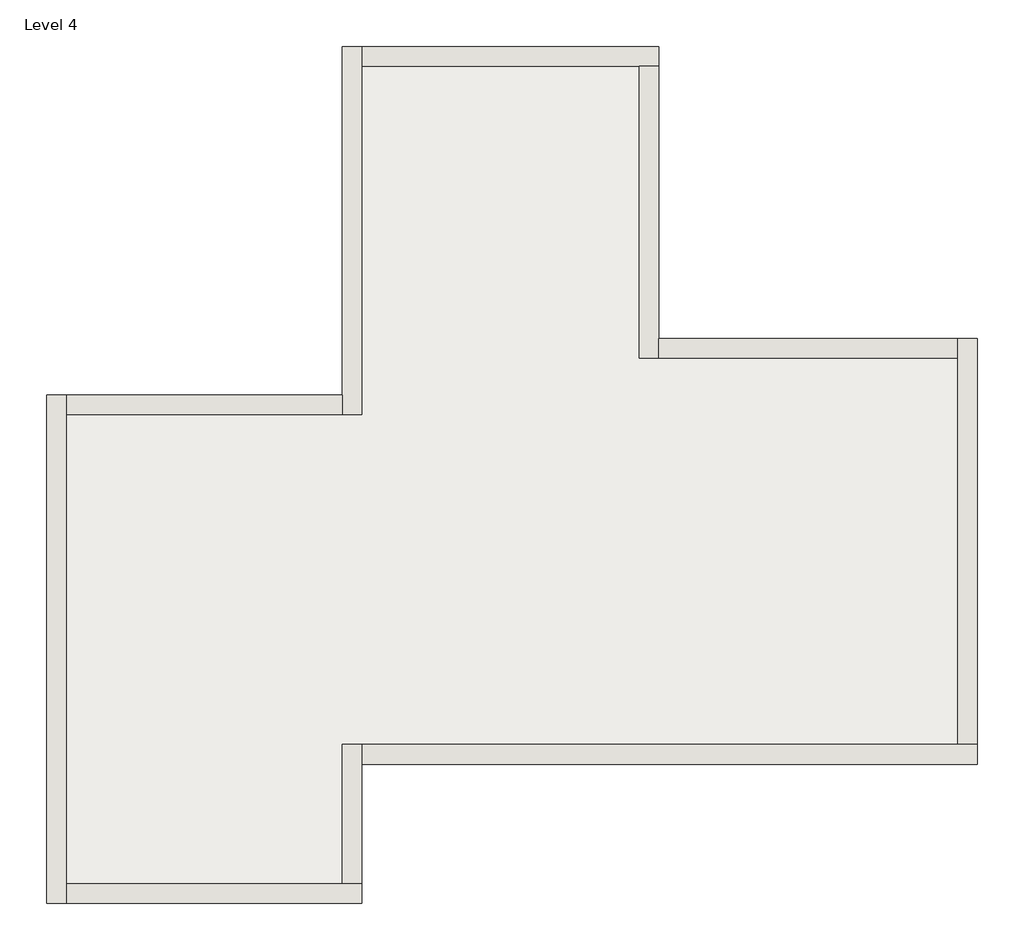
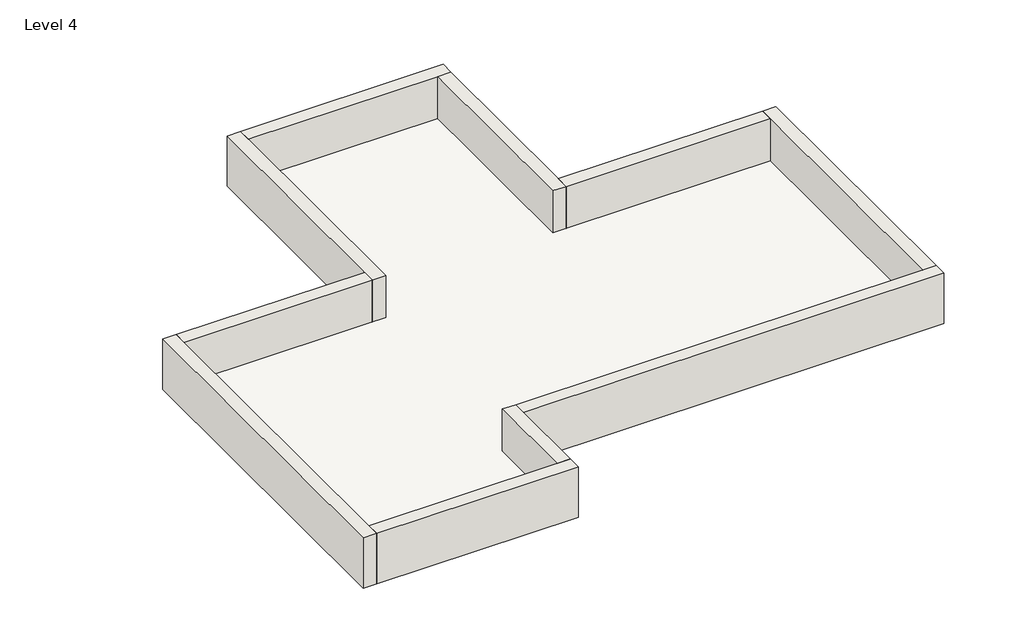
# One storey: 10 walls, 1 slab.
"""IFC4 building model written with IfcOpenShell, lengths in millimetres."""

from ifc_helpers import new_model, si_unit, frame, origin, place, context, project, spatial, polyline, outline, extrude, faceted_brep, element, save

model = new_model("IFC4")

# Units and contexts
model_context = context("Model", 3, world=origin())
ifc_project = project(units=[si_unit("LENGTHUNIT", "METRE", prefix="MILLI")], contexts=[model_context])

# Site, building, storey
site = spatial("IfcSite", under=ifc_project)
building = spatial("IfcBuilding", under=site)
storey = spatial("IfcBuildingStorey", under=building, Name="Level 4", Elevation=6705.6)

# Slab
placement = place(None, origin())
element("IfcSlab", 1, ObjectType="GENERIC 6\"", at=placement, inside=storey, context=model_context, shape_type="SweptSolid", body=[
    extrude(outline(polyline([(-5225.7431792, 1941.7051193), (-5225.7431792, -1474.5948807), (-1497.3206632, -1474.5948807), (-1497.3206632, -5995.7948807), (-8698.2206632, -5995.7948807), (-8698.2206632, -7621.3948807), (-11924.0206632, -7621.3948807), (-11924.0206632, -2134.9948807), (-8469.6206632, -2134.9948807), (-8469.6206632, 1941.7051193), (-5225.7431792, 1941.7051193)])), frame((0.0, 0.0, 6705.6), z_axis=(0.0, 0.0, 1.0), x_axis=(1.0, 0.0, 0.0)), (0.0, 0.0, 1.0), 152.4),
])

# Walls
element("IfcWall", 2, ObjectType="WALL 9\"", at=placement, inside=storey, context=model_context, shape_type="Brep", body=[
    faceted_brep([(-8469.6206632, -2134.9948807, 6705.6), (-8469.6206632, 1941.7051193, 6705.6), (-8469.6206632, 2170.3051193, 6705.6), (-8469.6206632, 2170.3051193, 7620.0), (-8469.6206632, 1941.7051193, 7620.0), (-8469.6206632, -2134.9948807, 7620.0), (-8698.2206632, -2134.9948807, 6705.6), (-8698.2206632, -2134.9948807, 7620.0), (-8698.2206632, -1906.3948807, 7620.0), (-8698.2206632, 2170.3051193, 7620.0), (-8698.2206632, 2170.3051193, 6705.6), (-8698.2206632, -1906.3948807, 6705.6)], [[[0, 1, 2, 3, 4, 5]], [[6, 7, 8, 9, 10, 11]], [[2, 1, 0, 6, 11, 10]], [[5, 4, 3, 9, 8, 7]], [[3, 2, 10, 9]], [[0, 5, 7, 6]]]),
])
element("IfcWall", 3, ObjectType="WALL 9\"", at=placement, inside=storey, context=model_context, shape_type="Brep", body=[
    faceted_brep([(-8469.6206632, 1941.7051193, 6705.6), (-5225.7431792, 1941.7051193, 6705.6), (-4997.1431792, 1941.7051193, 6705.6), (-4997.1431792, 1941.7051193, 7620.0), (-5225.7431792, 1941.7051193, 7620.0), (-8469.6206632, 1941.7051193, 7620.0), (-8469.6206632, 2170.3051193, 6705.6), (-8469.6206632, 2170.3051193, 7620.0), (-4997.1431792, 2170.3051193, 7620.0), (-4997.1431792, 2170.3051193, 6705.6)], [[[0, 1, 2, 3, 4, 5]], [[6, 7, 8, 9]], [[2, 1, 0, 6, 9]], [[5, 4, 3, 8, 7]], [[0, 5, 7, 6]], [[3, 2, 9, 8]]]),
])
element("IfcWall", 4, ObjectType="WALL 9\"", at=placement, inside=storey, context=model_context, shape_type="Brep", body=[
    faceted_brep([(-5225.7431792, 1941.7051193, 6705.6), (-5225.7431792, -1474.5948807, 6705.6), (-5225.7431792, -1474.5948807, 7620.0), (-5225.7431792, 1941.7051193, 7620.0), (-4997.1431792, 1941.7051193, 6705.6), (-4997.1431792, 1941.7051193, 7620.0), (-4997.1431792, -1245.9948807, 7620.0), (-4997.1431792, -1474.5948807, 7620.0), (-4997.1431792, -1474.5948807, 6705.6), (-4997.1431792, -1245.9948807, 6705.6)], [[[0, 1, 2, 3]], [[4, 5, 6, 7, 8, 9]], [[1, 0, 4, 9, 8]], [[3, 2, 7, 6, 5]], [[0, 3, 5, 4]], [[2, 1, 8, 7]]]),
])
element("IfcWall", 5, ObjectType="WALL 9\"", at=placement, inside=storey, context=model_context, shape_type="SweptSolid", body=[
    extrude(outline(polyline([(-11924.0206632, -1906.3948807), (-8698.2206632, -1906.3948807), (-8698.2206632, -2134.9948807), (-11924.0206632, -2134.9948807), (-11924.0206632, -1906.3948807)])), frame((0.0, 0.0, 6705.6), z_axis=(0.0, 0.0, 1.0), x_axis=(1.0, 0.0, 0.0)), (0.0, 0.0, 1.0), 914.4),
])
element("IfcWall", 6, ObjectType="WALL 9\"", at=placement, inside=storey, context=model_context, shape_type="Brep", body=[
    faceted_brep([(-12152.6206632, -1906.3948807, 6705.6), (-12152.6206632, -7849.9948807, 6705.6), (-12152.6206632, -7849.9948807, 7620.0), (-12152.6206632, -1906.3948807, 7620.0), (-11924.0206632, -1906.3948807, 6705.6), (-11924.0206632, -1906.3948807, 7620.0), (-11924.0206632, -2134.9948807, 7620.0), (-11924.0206632, -7621.3948807, 7620.0), (-11924.0206632, -7849.9948807, 7620.0), (-11924.0206632, -7849.9948807, 6705.6), (-11924.0206632, -7621.3948807, 6705.6), (-11924.0206632, -2134.9948807, 6705.6)], [[[0, 1, 2, 3]], [[4, 5, 6, 7, 8, 9, 10, 11]], [[1, 0, 4, 11, 10, 9]], [[3, 2, 8, 7, 6, 5]], [[2, 1, 9, 8]], [[0, 3, 5, 4]]]),
])
element("IfcWall", 7, ObjectType="WALL 9\"", at=placement, inside=storey, context=model_context, shape_type="Brep", body=[
    faceted_brep([(-8469.6206632, -7621.3948807, 6705.6), (-8698.2206632, -7621.3948807, 6705.6), (-11924.0206632, -7621.3948807, 6705.6), (-11924.0206632, -7621.3948807, 7620.0), (-8698.2206632, -7621.3948807, 7620.0), (-8469.6206632, -7621.3948807, 7620.0), (-8469.6206632, -7849.9948807, 6705.6), (-8469.6206632, -7849.9948807, 7620.0), (-11924.0206632, -7849.9948807, 7620.0), (-11924.0206632, -7849.9948807, 6705.6)], [[[0, 1, 2, 3, 4, 5]], [[6, 7, 8, 9]], [[2, 1, 0, 6, 9]], [[5, 4, 3, 8, 7]], [[3, 2, 9, 8]], [[0, 5, 7, 6]]]),
])
element("IfcWall", 8, ObjectType="WALL 9\"", at=placement, inside=storey, context=model_context, shape_type="Brep", body=[
    faceted_brep([(-8698.2206632, -5995.7948807, 6705.6), (-8698.2206632, -7621.3948807, 6705.6), (-8698.2206632, -7621.3948807, 7620.0), (-8698.2206632, -5995.7948807, 7620.0), (-8469.6206632, -5995.7948807, 6705.6), (-8469.6206632, -5995.7948807, 7620.0), (-8469.6206632, -6224.3948807, 7620.0), (-8469.6206632, -7621.3948807, 7620.0), (-8469.6206632, -7621.3948807, 6705.6), (-8469.6206632, -6224.3948807, 6705.6)], [[[0, 1, 2, 3]], [[4, 5, 6, 7, 8, 9]], [[1, 0, 4, 9, 8]], [[3, 2, 7, 6, 5]], [[2, 1, 8, 7]], [[0, 3, 5, 4]]]),
])
element("IfcWall", 9, ObjectType="WALL 9\"", at=placement, inside=storey, context=model_context, shape_type="Brep", body=[
    faceted_brep([(-1268.7206632, -5995.7948807, 6705.6), (-1497.3206632, -5995.7948807, 6705.6), (-8469.6206632, -5995.7948807, 6705.6), (-8469.6206632, -5995.7948807, 7620.0), (-1497.3206632, -5995.7948807, 7620.0), (-1268.7206632, -5995.7948807, 7620.0), (-1268.7206632, -6224.3948807, 6705.6), (-1268.7206632, -6224.3948807, 7620.0), (-8469.6206632, -6224.3948807, 7620.0), (-8469.6206632, -6224.3948807, 6705.6)], [[[0, 1, 2, 3, 4, 5]], [[6, 7, 8, 9]], [[2, 1, 0, 6, 9]], [[5, 4, 3, 8, 7]], [[3, 2, 9, 8]], [[0, 5, 7, 6]]]),
])
element("IfcWall", 10, ObjectType="WALL 9\"", at=placement, inside=storey, context=model_context, shape_type="Brep", body=[
    faceted_brep([(-1268.7206632, -5995.7948807, 6705.6), (-1268.7206632, -1245.9948807, 6705.6), (-1268.7206632, -1245.9948807, 7620.0), (-1268.7206632, -5995.7948807, 7620.0), (-1497.3206632, -5995.7948807, 6705.6), (-1497.3206632, -5995.7948807, 7620.0), (-1497.3206632, -1474.5948807, 7620.0), (-1497.3206632, -1245.9948807, 7620.0), (-1497.3206632, -1245.9948807, 6705.6), (-1497.3206632, -1474.5948807, 6705.6)], [[[0, 1, 2, 3]], [[4, 5, 6, 7, 8, 9]], [[1, 0, 4, 9, 8]], [[3, 2, 7, 6, 5]], [[0, 3, 5, 4]], [[2, 1, 8, 7]]]),
])
element("IfcWall", 11, ObjectType="WALL 9\"", at=placement, inside=storey, context=model_context, shape_type="SweptSolid", body=[
    extrude(outline(polyline([(-4997.1431792, -1245.9948807), (-1497.3206632, -1245.9948807), (-1497.3206632, -1474.5948807), (-4997.1431792, -1474.5948807), (-4997.1431792, -1245.9948807)])), frame((0.0, 0.0, 6705.6), z_axis=(0.0, 0.0, 1.0), x_axis=(1.0, 0.0, 0.0)), (0.0, 0.0, 1.0), 914.4),
])

save(model, "model.ifc")

# Revit data of these elements
# Type "GENERIC 6\""
#   Assembly Code = "B1010"
#   Function = 0
#   Layers, outside or top first: 0' - 6" no material (function 1)
# Type "WALL 9\""
#   Assembly Code = "B2010"
#   Layers, outside or top first: 0' - 9" "SOFT COOL PAINT" (function 1)
# Element 1 (IfcSlab, "GENERIC 6\"")
#   Height Offset From Level = 0' - 6"
#   Phase Created = New Construction
#   Materials on its faces: "Default Floor"
# Elements 2, 3, 4, 5, 6, 7, 8, 9, 10, 11 (IfcWall, "WALL 9\"")
#   Top Offset = 0' - 0"
#   Base Offset = 0' - 0"
#   Unconnected Height = 3' - 0"
#   wall height = 3' - 0"
#   Phase Created = New Construction
#   Base Constraint = Level 4
#   Materials on its faces: "SOFT COOL PAINT"
# Materials
#   "SOFT COOL PAINT": class "Generic", colour RGB 120 120 120, transparency 0, Cost = 0
#   "Default Floor": colour RGB 128 128 128, transparency 0, Cost = 0
